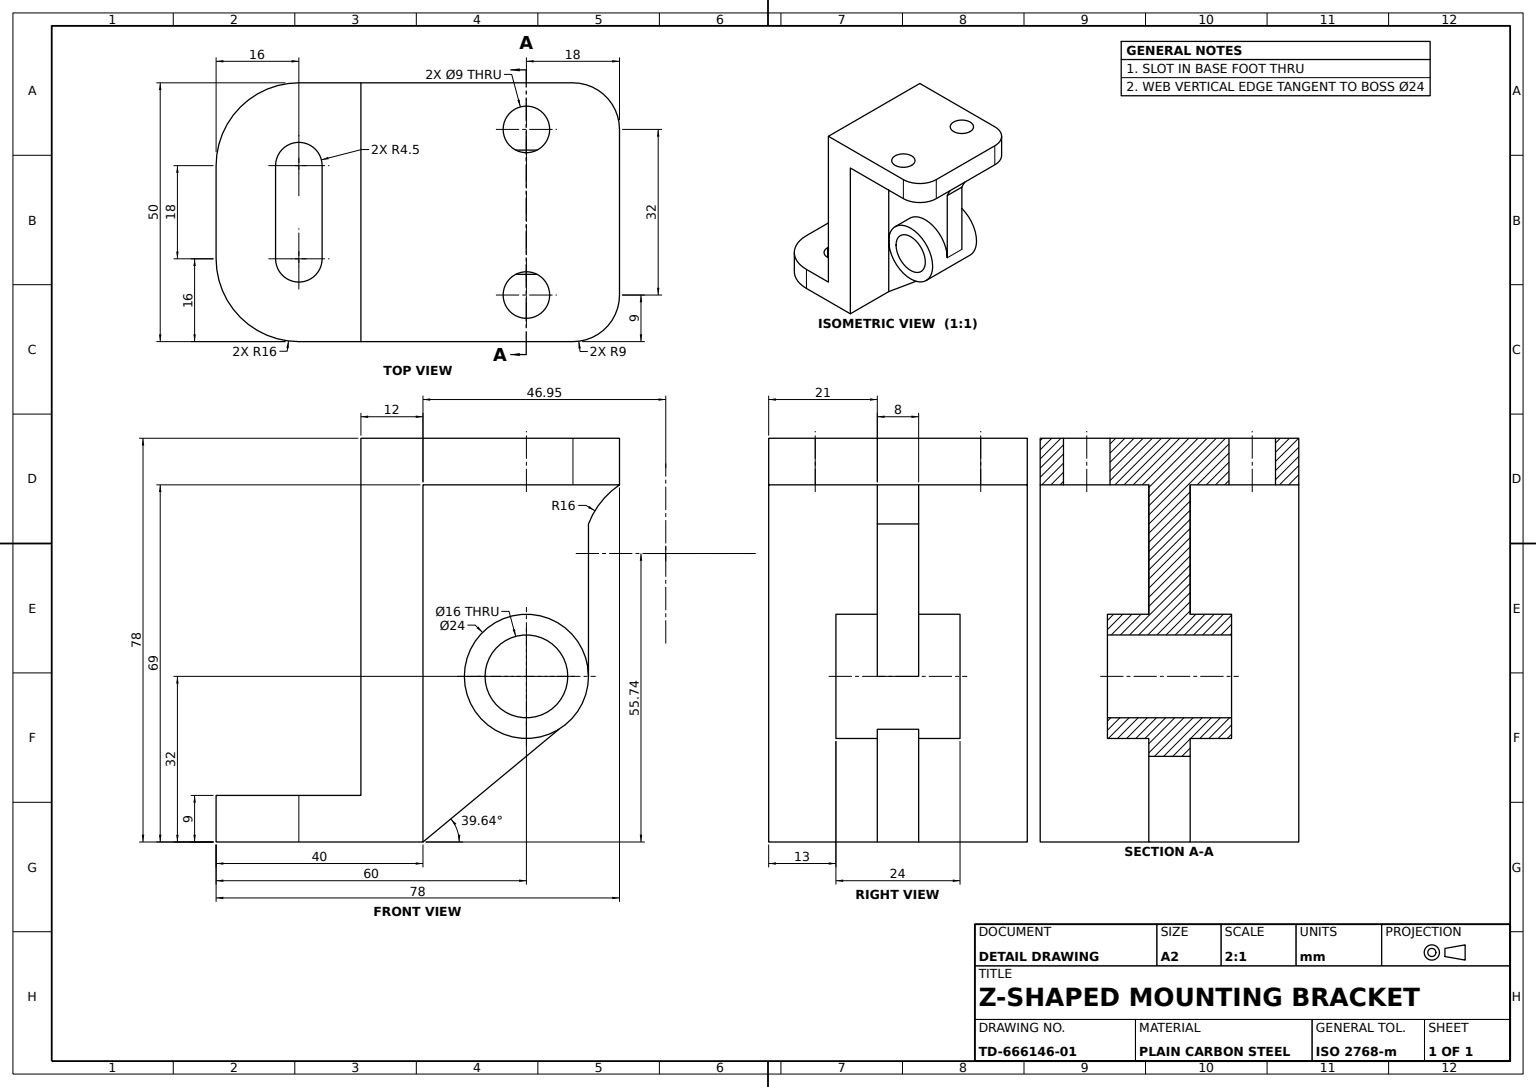
from build123d import *
from build123d.topology import SkipClean

# Parameters (mm, degrees)
BASE_FOOT_WITH_SLOT_DEPTH     = 9
UPRIGHT_WALL_SKETCH_W         = 50
UPRIGHT_WALL_SKETCH_H         = 69
UPRIGHT_WALL_DEPTH            = 12
TOP_FLANGE_SKETCH_R           = 4.5
TOP_FLANGE_WITH_2_HOLES_DEPTH = 9
SIDE_BOSS_SKETCH_R            = 12
SIDE_BOSS_SKETCH_R_2          = 8
SIDE_BOSS_DEPTH               = 12
BOSS_WEB_DEPTH                = 4
BOSS_BORE_SKETCH_R            = 8
BOSS_BORE_DEPTH               = 102.434708064


with BuildPart() as part:
    # Base Foot Sketch → Base Foot with Slot (new body)
    with BuildSketch(Plane(origin=(0, 0, 0), x_dir=(1, 0, 0), z_dir=(0, 1, 0))):
        with BuildLine():
            Line((-25, 20), (25, 20))
            Line((25, 20), (25, -4))
            ThreePointArc((25, -4), (20.313708499, -15.313708499), (9, -20))
            Line((9, -20), (-9, -20))
            ThreePointArc((-9, -20), (-20.313708499, -15.313708499), (-25, -4))
            Line((-25, -4), (-25, 20))
        make_face()
        with BuildLine():
            Line((-9, 0.5), (9, 0.5))
            ThreePointArc((9, 0.5), (13.5, -4), (9, -8.5))
            Line((9, -8.5), (-9, -8.5))
            ThreePointArc((-9, -8.5), (-13.5, -4), (-9, 0.5))
        make_face(mode=Mode.SUBTRACT)
    extrude(amount=BASE_FOOT_WITH_SLOT_DEPTH)

    # Upright Wall Sketch → Upright Wall (add)
    with BuildSketch(Plane(origin=(0, 0, -20), x_dir=(-1, 0, 0), z_dir=(0, 0, -1))):
        with Locations((0, 43.5)):
            Rectangle(UPRIGHT_WALL_SKETCH_W, UPRIGHT_WALL_SKETCH_H)
    extrude(amount=-UPRIGHT_WALL_DEPTH)

    # Top Flange Sketch → Top Flange with 2 Holes (add)
    with BuildSketch(Plane(origin=(0, 78, 0), x_dir=(1, 0, 0), z_dir=(0, 1, 0))):
        with BuildLine():
            Line((-25, 20), (-25, 49))
            ThreePointArc((-25, 49), (-22.363961031, 55.363961031), (-16, 58))
            Line((-16, 58), (16, 58))
            ThreePointArc((16, 58), (22.363961031, 55.363961031), (25, 49))
            Line((25, 49), (25, 20))
            Line((25, 20), (-25, 20))
        make_face()
        with Locations(Location((-16, 40, 0), (0, 0, 270))):
            Circle(TOP_FLANGE_SKETCH_R, mode=Mode.SUBTRACT)
        with Locations(Location((16, 40, 0), (0, 0, 270))):
            Circle(TOP_FLANGE_SKETCH_R, mode=Mode.SUBTRACT)
    extrude(amount=-TOP_FLANGE_WITH_2_HOLES_DEPTH)



with BuildPart() as body_2:
    # Side Boss Sketch → Side Boss (new, symmetric)
    with BuildSketch(Plane(origin=(0, 0, 0), x_dir=(0, 0, -1), z_dir=(1, 0, 0))):
        with Locations((40, 32)):
            Circle(SIDE_BOSS_SKETCH_R)
        with Locations((40, 32)):
            Circle(SIDE_BOSS_SKETCH_R_2, mode=Mode.SUBTRACT)
    extrude(amount=SIDE_BOSS_DEPTH, both=True)


with BuildPart() as part_1:
    with SkipClean():  # the faces are left unmerged after this step: merging them gives an invalid solid
        add(part.part)

        add(body_2.part)  # Boss Web merges body 2
        # Boss Web Sketch → Boss Web (add, symmetric)
        with BuildSketch(Plane(origin=(0, 0, 0), x_dir=(0, 0, -1), z_dir=(1, 0, 0))):
            with BuildLine():
                Line((52, 32), (52, 61.444590884))
                ThreePointArc((52, 61.444590884), (54.416944157, 65.68531935), (58, 69))
                Line((58, 69), (20, 69))
                Line((20, 69), (20, 0))
                Line((20, 0), (46.285769513, 21.778008921))
                ThreePointArc((46.285769513, 21.778008921), (50.474474549, 26.144627858), (52, 32))
            make_face()
        extrude(amount=BOSS_WEB_DEPTH, both=True)

    # Boss Bore Sketch → Boss Bore (cut, through all)
    with SkipClean():  # the faces are left unmerged after this step: merging them gives an invalid solid
        with BuildSketch(Plane.ZY.offset(4)):
            with Locations(Location((-40, 32, 0), (0, 0, 180))):
                Circle(BOSS_BORE_SKETCH_R)
        extrude(amount=-BOSS_BORE_DEPTH, mode=Mode.SUBTRACT)


solid = part_1.part
